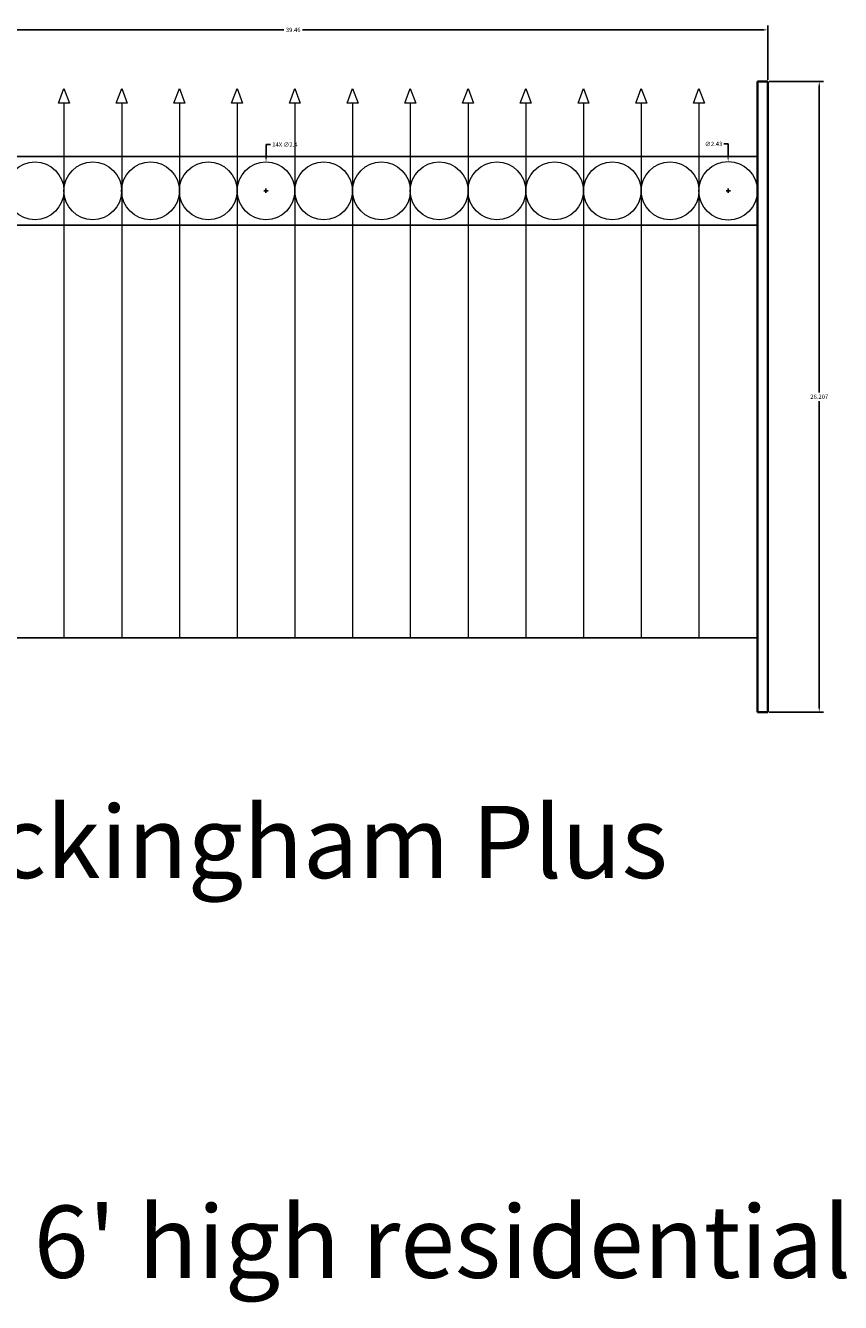
# Model space of a CAD drawing. Units: inches. Extents: x 756 to 915, y 488 to 695.
# Tile 2 of 25: x 779 to 813, y 488 to 541. Entities that reach past the tile are written whole.
import ezdxf

# ---------------------------------------------------------------- set-up
doc = ezdxf.new("R2010")
doc.units = ezdxf.units.IN
doc.header["$MEASUREMENT"] = 0
for name, color, linetype, lineweight in [('L-ANNO-TEXT', 7, 'Continuous', 25), ('L-FENC-PCKT', 7, 'Continuous', 18), ('L-FENC-POST', 7, 'Continuous', 35), ('L-FENC-RAIL', 7, 'Continuous', 25), ('L-FENC-RING', 7, 'Continuous', 18), ('M-DIMS', 2, 'Continuous', 18)]:
    doc.layers.add(name, color=color, linetype=linetype, lineweight=lineweight)
doc.styles.get("Standard").update_dxf_attribs({"font": 'arial.ttf'})
doc.dimstyles.get("Standard").update_dxf_attribs({"dimtxt": 0.18, "dimasz": 0.18, "dimexe": 0.18, "dimexo": 0.0625, "dimgap": 0.09, "dimtad": 0, "dimtih": 1, "dimtoh": 1, "dimdec": 0, "dimzin": 0, "dimdsep": 46, "dimlunit": 3, "dimtxsty": 'Standard', "dimcen": 0.09, "dimadec": 0, "dimazin": 0, "dimtfac": 1, "dimtdec": 0, "dimtofl": 0, "dimtmove": 0, "dimatfit": 3, "dimfxl": 1, "dimtolj": 1, "dimtzin": 0, "dimarcsym": 0})

# ---------------------------------------------------------------- blocks, each defined once
blk = doc.blocks.new('FENCE-POST-RIGHT')
for p, q in [((0, 26.207), (0, 0)), ((0, 26.207), (0.427, 26.207)), ((0.427, 26.207), (0.427, 0)), ((0, 0), (0.427, 0))]:
    blk.add_line(p, q)
blk = doc.blocks.new('PICKET-SPEAR-FLUSH')
blk.add_line((0.228, 22.215), (0.228, 0))
blk.add_lwpolyline([(0.228, 22.215), (0, 22.215), (0.228, 22.826), (0.455, 22.215)], close=True)
blk = doc.blocks.new('FENCE-PLUS-RING-BAND')
for centre, radius in [((1.286, 1.286), 1.286), ((3.773, 1.286), 1.2), ((6.173, 1.286), 1.2), ((8.572, 1.286), 1.2), ((10.972, 1.286), 1.2), ((13.372, 1.286), 1.2), ((15.772, 1.286), 1.2), ((18.172, 1.286), 1.2), ((20.572, 1.286), 1.2), ((22.972, 1.286), 1.2), ((25.372, 1.286), 1.2), ((27.772, 1.286), 1.2), ((30.172, 1.286), 1.2), ((32.572, 1.286), 1.2), ((34.971, 1.286), 1.2), ((37.388, 1.286), 1.217)]:
    blk.add_circle(centre, radius)
blk = doc.blocks.new('*D72')
at = {"layer": 'Defpoints', "color": 0, "transparency": 16777216}
for p in [(810.347, 540.934), (770.889, 538.794), (810.347, 538.794)]:
    blk.add_point(p, dxfattribs=at)
at = {"layer": 'M-DIMS', "color": 0, "lineweight": -2, "transparency": 16777216}
for p, q in [((770.889, 538.857), (770.889, 541.114)), ((771.069, 540.934), (790.224, 540.934)), ((810.167, 540.934), (791.011, 540.934)), ((810.347, 538.857), (810.347, 541.114))]:
    blk.add_line(p, q, dxfattribs=at)
at = {"layer": 'M-DIMS', "color": 0, "transparency": 16777216}
for points in [[(771.069, 540.964), (771.069, 540.904), (770.889, 540.934)], [(810.167, 540.964), (810.167, 540.904), (810.347, 540.934)]]:
    blk.add_solid(points, dxfattribs=at)
at = {"layer": 'M-DIMS', "color": 0, "transparency": 16777216, "insert": (790.618, 540.934), "char_height": 0.18, "attachment_point": 5}
blk.add_mtext('\\A1;39.46', dxfattribs=at)
blk = doc.blocks.new('*D73')
at = {"layer": 'Defpoints', "color": 0, "transparency": 16777216}
for p in [(810.347, 538.794), (812.487, 538.794), (810.347, 512.587)]:
    blk.add_point(p, dxfattribs=at)
at = {"layer": 'M-DIMS', "color": 0, "lineweight": -2, "transparency": 16777216}
for p, q in [((810.409, 538.794), (812.667, 538.794)), ((812.487, 538.614), (812.487, 525.873)), ((812.487, 512.767), (812.487, 525.509)), ((810.409, 512.587), (812.667, 512.587))]:
    blk.add_line(p, q, dxfattribs=at)
at = {"layer": 'M-DIMS', "color": 0, "transparency": 16777216}
for points in [[(812.457, 538.614), (812.517, 538.614), (812.487, 538.794)], [(812.457, 512.767), (812.517, 512.767), (812.487, 512.587)]]:
    blk.add_solid(points, dxfattribs=at)
at = {"layer": 'M-DIMS', "color": 0, "transparency": 16777216, "insert": (812.487, 525.691), "char_height": 0.18, "attachment_point": 5}
blk.add_mtext('\\A1;26.207', dxfattribs=at)
blk = doc.blocks.new('*D85')
at = {"layer": 'Defpoints', "color": 0, "transparency": 16777216}
for p in [(789.49, 535.447), (789.484, 533.047)]:
    blk.add_point(p, dxfattribs=at)
at = {"layer": 'M-DIMS', "color": 0, "lineweight": -2, "transparency": 16777216}
for p, q in [((789.492, 536.167), (789.49, 535.627)), ((789.672, 536.167), (789.492, 536.167)), ((789.487, 534.157), (789.487, 534.337)), ((789.397, 534.247), (789.577, 534.247))]:
    blk.add_line(p, q, dxfattribs=at)
at = {"layer": 'M-DIMS', "color": 0, "transparency": 16777216}
blk.add_solid([(789.46, 535.627), (789.52, 535.627), (789.49, 535.447)], dxfattribs=at)
at = {"layer": 'M-DIMS', "color": 0, "transparency": 16777216, "insert": (790.273, 536.167), "char_height": 0.18, "attachment_point": 5}
blk.add_mtext('\\A1;14X ∅2.4', dxfattribs=at)
blk = doc.blocks.new('*D86')
at = {"layer": 'Defpoints', "color": 0, "transparency": 16777216}
for p in [(808.7, 535.464), (808.706, 533.03)]:
    blk.add_point(p, dxfattribs=at)
at = {"layer": 'M-DIMS', "color": 0, "lineweight": -2, "transparency": 16777216}
for p, q in [((808.518, 536.194), (808.698, 536.194)), ((808.698, 536.194), (808.7, 535.644)), ((808.703, 534.157), (808.703, 534.337)), ((808.613, 534.247), (808.793, 534.247))]:
    blk.add_line(p, q, dxfattribs=at)
at = {"layer": 'M-DIMS', "color": 0, "transparency": 16777216}
blk.add_solid([(808.73, 535.644), (808.67, 535.644), (808.7, 535.464)], dxfattribs=at)
at = {"layer": 'M-DIMS', "color": 0, "transparency": 16777216, "insert": (808.096, 536.194), "char_height": 0.18, "attachment_point": 5}
blk.add_mtext('\\A1;∅2.43', dxfattribs=at)

msp = doc.modelspace()

# ---------------------------------------------------------------- linework, layer by layer
at = {"layer": 'L-FENC-RAIL'}
for p, q in [((771.3152, 535.6792), (809.92, 535.6792)), ((771.3152, 532.8149), (809.92, 532.8149)), ((771.3152, 515.6691), (809.92, 515.6691))]:
    msp.add_line(p, q, dxfattribs=at)

# ---------------------------------------------------------------- block references
at = {"layer": 'L-FENC-PCKT'}
for p in [(780.8597, 515.6687), (783.2596, 515.6687), (785.6596, 515.6687), (788.0595, 515.6687), (790.4594, 515.6687), (792.8593, 515.6687), (795.2592, 515.6687), (797.6591, 515.6687), (800.059, 515.6687), (802.4589, 515.6687), (804.8588, 515.6687), (807.2588, 515.6687)]:
    msp.add_blockref('PICKET-SPEAR-FLUSH', p, dxfattribs=at)
at = {"layer": 'L-FENC-POST', "rotation": 180}
msp.add_blockref('FENCE-POST-RIGHT', (810.3468, 538.7943), dxfattribs=at)
at = {"layer": 'L-FENC-RING'}
msp.add_blockref('FENCE-PLUS-RING-BAND', (771.315, 532.961), dxfattribs=at)

# ---------------------------------------------------------------- texts
at = {"layer": 'L-ANNO-TEXT'}
for s, p in [('Buckingham Plus', (773.0883, 505.6907)), ("6' high residential fences have four horizontal rails, not three as shown.", (779.8362, 489.0819))]:
    msp.add_text(s, height=3, dxfattribs=at).set_placement(p)

# ---------------------------------------------------------------- dimensions: what is measured, and where the dimension line sits
at = {"layer": 'M-DIMS'}
dim = msp.add_linear_dim(base=(810.3467, 540.9342), p1=(770.8885, 538.7942), p2=(810.3467, 538.7942), dimstyle='Standard', override={"dimdec": 2, "dimlfac": 1, "dimrnd": 0, "dimzin": 0, "dimdsep": 46, "dimlunit": 2}, dxfattribs=at)
dim.commit()
dim.dimension.update_dxf_attribs({"geometry": '*D72', "text_midpoint": (790.6176, 540.9342)})
dim = msp.add_linear_dim(base=(812.4867, 538.7942), p1=(810.3467, 512.5874), p2=(810.3467, 538.7942), angle=90, dimstyle='Standard', override={"dimdec": 3, "dimlfac": 1, "dimrnd": 0, "dimzin": 0, "dimdsep": 46, "dimlunit": 2}, dxfattribs=at)
dim.commit()
dim.dimension.update_dxf_attribs({"geometry": '*D73', "text_midpoint": (812.4867, 525.6908)})
dim = msp.add_diameter_dim_2p(p1=(789.4841, 533.0471), p2=(789.49, 535.447), text='14X <>', dimstyle='Standard', override={"dimdec": 1, "dimlfac": 1, "dimrnd": 0, "dimzin": 0, "dimdsep": 46, "dimlunit": 2}, dxfattribs=at)
dim.commit()
dim.dimension.update_dxf_attribs({"geometry": '*D85', "text_midpoint": (790.2732, 536.167), "dimtype": 163})
dim = msp.add_diameter_dim_2p(p1=(808.7064, 533.0303), p2=(808.7, 535.4639), dimstyle='Standard', override={"dimdec": 2, "dimlfac": 1, "dimrnd": 0, "dimzin": 0, "dimdsep": 46, "dimlunit": 2}, dxfattribs=at)
dim.commit()
dim.dimension.update_dxf_attribs({"geometry": '*D86', "text_midpoint": (808.0964, 536.1939), "dimtype": 163})

doc.saveas('drawing.dxf')
